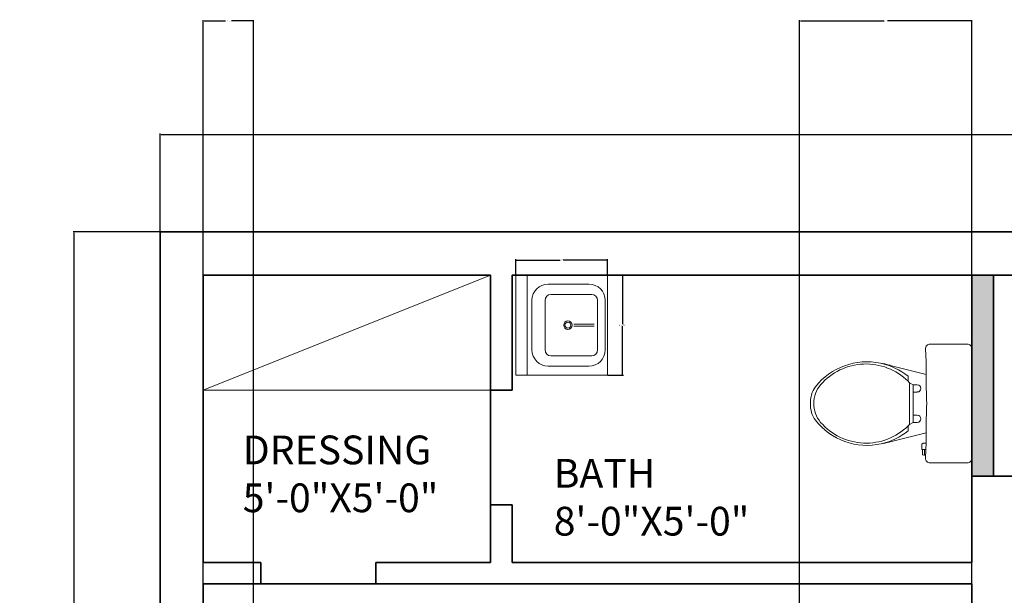
# Model space of a CAD drawing. Units: inches. Extents: x -10 to 502, y -868 to 56.
# Tile 11 of 14: x 6 to 211, y -64 to 56. Entities that reach past the tile are written whole.
import ezdxf

# ---------------------------------------------------------------- set-up
doc = ezdxf.new("R2010")
doc.units = ezdxf.units.IN
doc.header["$MEASUREMENT"] = 0
for name, color, linetype, lineweight in [('A-ANNO-DIMS', 2, 'Continuous', 18), ('A-AREA-IDEN', 7, 'Continuous', 18), ('A-FLOR-CASE', 8, 'Continuous', 18), ('A-FLOR-FIXT', 8, 'Continuous', 18), ('A-WALL', 7, 'Continuous', 35), ('A-WALL-PATT', 5, 'Continuous', 13), ('WC-Detail_dwgmodels.com', 251, 'Continuous', 13), ('WC-Outline_dwgmodels.com', 250, 'Continuous', 18)]:
    doc.layers.add(name, color=color, linetype=linetype, lineweight=lineweight)
doc.styles.get("Standard").update_dxf_attribs({"font": 'arial.ttf'})
doc.dimstyles.get("Standard").update_dxf_attribs({"dimtxt": 0.18, "dimasz": 0.18, "dimexe": 0.18, "dimexo": 0.0625, "dimgap": 0.09, "dimtad": 0, "dimtih": 1, "dimtoh": 1, "dimdec": 0, "dimzin": 0, "dimdsep": 46, "dimlunit": 3, "dimtxsty": 'Standard', "dimcen": 0.09, "dimadec": 0, "dimazin": 0, "dimtfac": 1, "dimtdec": 0, "dimtofl": 0, "dimtmove": 0, "dimatfit": 3, "dimfxl": 1, "dimtolj": 1, "dimtzin": 0, "dimarcsym": 0})

# ---------------------------------------------------------------- blocks, each defined once
blk = doc.blocks.new('*D1')
at = {"layer": 'A-ANNO-DIMS', "color": 0, "lineweight": -2, "transparency": 16777216}
for p, q in [((34.95, 12.21), (34.95, 32.67)), ((35.13, 32.49), (236.06, 32.49)), ((457.77, 32.49), (256.84, 32.49)), ((457.95, 12.21), (457.95, 32.67))]:
    blk.add_line(p, q, dxfattribs=at)
at = {"layer": 'A-ANNO-DIMS', "color": 0, "transparency": 16777216}
for points in [[(35.13, 32.52), (35.13, 32.46), (34.95, 32.49)], [(457.77, 32.52), (457.77, 32.46), (457.95, 32.49)]]:
    blk.add_solid(points, dxfattribs=at)
at = {"layer": 'Defpoints', "color": 0, "transparency": 16777216}
for p in [(457.95, 32.49), (34.95, 12.15), (457.95, 12.15)]:
    blk.add_point(p, dxfattribs=at)
at = {"layer": 'A-ANNO-DIMS', "color": 0, "transparency": 16777216, "insert": (246.45, 32.49), "char_height": 6, "attachment_point": 5}
blk.add_mtext('\\A1;35\'-3"', dxfattribs=at)
blk = doc.blocks.new('*D2')
at = {"layer": 'A-ANNO-DIMS', "color": 0, "lineweight": -2, "transparency": 16777216}
for p, q in [((34.89, 12.15), (16.75, 12.15)), ((16.93, 11.97), (16.93, -376.2)), ((16.93, -770.67), (16.93, -382.51)), ((34.89, -770.85), (16.75, -770.85))]:
    blk.add_line(p, q, dxfattribs=at)
at = {"layer": 'A-ANNO-DIMS', "color": 0, "transparency": 16777216}
for points in [[(16.9, 11.97), (16.96, 11.97), (16.93, 12.15)], [(16.9, -770.67), (16.96, -770.67), (16.93, -770.85)]]:
    blk.add_solid(points, dxfattribs=at)
at = {"layer": 'Defpoints', "color": 0, "transparency": 16777216}
for p in [(34.95, 12.15), (16.93, -770.85), (34.95, -770.85)]:
    blk.add_point(p, dxfattribs=at)
at = {"layer": 'A-ANNO-DIMS', "color": 0, "transparency": 16777216, "insert": (16.93, -379.35), "char_height": 6, "attachment_point": 5}
blk.add_mtext('\\A1;65\'-3"', dxfattribs=at)
blk = doc.blocks.new('М14 600х655')
for p, q in [((-655, 600), (-655, 0)), ((-655, 600), (-655, 0)), ((-655, 0), (-655, 600)), ((0, 600), (-655, 600)), ((0, 0), (0, 600)), ((0, 525), (-655, 525)), ((-165.1, 494.1), (-489.9, 494.1)), ((-595.8, 388.1), (-595.8, 121.3)), ((-165.4, 408.4), (-490.2, 408.4)), ((-59.2, 121.3), (-59.2, 388.1)), ((-528.4, 370.1), (-528.4, 103.3)), ((-127.2, 103.3), (-127.2, 370.1)), ((-333.5, 87.1), (-333.5, 219.6)), ((-321.5, 87.1), (-321.5, 219.6)), ((-490.2, 65.1), (-165.4, 65.1)), ((-655, 0), (-655, 0)), ((-655, 0), (-655, 0)), ((-655, 0), (0, 0)), ((-655, 0), (0, 0)), ((-489.9, 15.4), (-165.1, 15.4))]:
    blk.add_line(p, q)
for radius in [27.6, 19.3]:
    blk.add_circle((-327.5, 258.9), radius)
for centre, radius, start, end in [((-489.9, 388.1), 105.9, 90, 180), ((-165.1, 388.1), 105.9, 0, 90), ((-490.2, 370.1), 38.2, 90, 180), ((-165.4, 370.1), 38.2, 0, 90), ((-489.9, 121.3), 105.9, 180, 270), ((-490.2, 103.3), 38.2, 180, 270), ((-165.4, 103.3), 38.2, 270, 0), ((-165.1, 121.3), 105.9, 270, 0)]:
    blk.add_arc(centre, radius, start, end)
blk = doc.blocks.new('*D29')
at = {"layer": 'A-ANNO-DIMS', "color": 0, "lineweight": -2, "transparency": 16777216}
for p, q in [((128.41, 3.15), (131.66, 3.15)), ((131.48, 2.97), (131.48, -7.12)), ((131.48, -17.58), (131.48, -7.49)), ((128.41, -17.76), (131.66, -17.76))]:
    blk.add_line(p, q, dxfattribs=at)
at = {"layer": 'A-ANNO-DIMS', "color": 0, "transparency": 16777216}
for points in [[(131.45, 2.97), (131.51, 2.97), (131.48, 3.15)], [(131.45, -17.58), (131.51, -17.58), (131.48, -17.76)]]:
    blk.add_solid(points, dxfattribs=at)
at = {"layer": 'Defpoints', "color": 0, "transparency": 16777216}
for p in [(128.35, 3.15), (131.48, 3.15), (128.35, -17.76)]:
    blk.add_point(p, dxfattribs=at)
at = {"layer": 'A-ANNO-DIMS', "color": 0, "transparency": 16777216, "insert": (131.48, -7.31), "char_height": 0.18, "attachment_point": 5}
blk.add_mtext('\\A1;BASIN 1\'-9"', dxfattribs=at)
blk = doc.blocks.new('*D30')
at = {"layer": 'A-ANNO-DIMS', "color": 0, "lineweight": -2, "transparency": 16777216}
for p, q in [((109.2, 3.21), (109.2, 6.46)), ((109.38, 6.28), (118.45, 6.28)), ((128.17, 6.28), (119.09, 6.28)), ((128.35, 3.21), (128.35, 6.46))]:
    blk.add_line(p, q, dxfattribs=at)
at = {"layer": 'A-ANNO-DIMS', "color": 0, "transparency": 16777216}
for points in [[(109.38, 6.31), (109.38, 6.25), (109.2, 6.28)], [(128.17, 6.31), (128.17, 6.25), (128.35, 6.28)]]:
    blk.add_solid(points, dxfattribs=at)
at = {"layer": 'Defpoints', "color": 0, "transparency": 16777216}
for p in [(109.2, 6.28), (109.2, 3.15), (128.35, 3.15)]:
    blk.add_point(p, dxfattribs=at)
at = {"layer": 'A-ANNO-DIMS', "color": 0, "transparency": 16777216, "insert": (118.77, 6.28), "char_height": 0.18, "attachment_point": 5}
blk.add_mtext('\\A1;1\'-7"', dxfattribs=at)
blk = doc.blocks.new('*D60')
at = {"layer": 'A-ANNO-DIMS', "color": 0, "lineweight": -2, "transparency": 16777216}
for p, q in [((168.45, -332.79), (168.45, 56.38)), ((168.63, 56.2), (186.12, 56.2)), ((204.27, 56.2), (186.78, 56.2)), ((204.45, -332.79), (204.45, 56.38))]:
    blk.add_line(p, q, dxfattribs=at)
at = {"layer": 'A-ANNO-DIMS', "color": 0, "transparency": 16777216}
for points in [[(168.63, 56.23), (168.63, 56.17), (168.45, 56.2)], [(204.27, 56.23), (204.27, 56.17), (204.45, 56.2)]]:
    blk.add_solid(points, dxfattribs=at)
at = {"layer": 'Defpoints', "color": 0, "transparency": 16777216}
for p in [(204.45, 56.2), (168.45, -332.85), (204.45, -332.85)]:
    blk.add_point(p, dxfattribs=at)
at = {"layer": 'A-ANNO-DIMS', "color": 0, "transparency": 16777216, "insert": (186.45, 56.2), "char_height": 0.18, "attachment_point": 5}
blk.add_mtext('\\A1;3\'-0"', dxfattribs=at)
blk = doc.blocks.new('*D64')
at = {"layer": 'A-ANNO-DIMS', "color": 0, "lineweight": -2, "transparency": 16777216}
for p, q in [((43.95, -332.79), (43.95, 56.38)), ((44.13, 56.2), (48.59, 56.2)), ((54.27, 56.2), (49.81, 56.2)), ((54.45, -332.79), (54.45, 56.38))]:
    blk.add_line(p, q, dxfattribs=at)
at = {"layer": 'A-ANNO-DIMS', "color": 0, "transparency": 16777216}
for points in [[(44.13, 56.23), (44.13, 56.17), (43.95, 56.2)], [(54.27, 56.23), (54.27, 56.17), (54.45, 56.2)]]:
    blk.add_solid(points, dxfattribs=at)
at = {"layer": 'Defpoints', "color": 0, "transparency": 16777216}
for p in [(54.45, 56.2), (43.95, -332.85), (54.45, -332.85)]:
    blk.add_point(p, dxfattribs=at)
at = {"layer": 'A-ANNO-DIMS', "color": 0, "transparency": 16777216, "insert": (49.2, 56.2), "char_height": 0.18, "attachment_point": 5}
blk.add_mtext('\\A1;0\'-10 1/2"', dxfattribs=at)

msp = doc.modelspace()

# ---------------------------------------------------------------- hatches: boundary and pattern name
at = {"layer": 'A-WALL-PATT'}
h = msp.add_hatch(color=256, dxfattribs=at)
h.dxf.hatch_style = 1
h.paths.add_polyline_path([(208.95, 3.15), (204.45, 3.15), (204.45, -38.85), (208.95, -38.85)])

# ---------------------------------------------------------------- linework, layer by layer
at = {"layer": 'A-FLOR-CASE'}
for p, q in [((103.95, 3.15), (43.95, -20.85)), ((43.95, -20.85), (103.95, -20.85))]:
    msp.add_line(p, q, dxfattribs=at)
at = {"layer": 'A-WALL'}
for p, q in [((34.95, 12.15), (34.95, -770.85)), ((34.95, 12.15), (457.95, 12.15)), ((43.95, 3.15), (43.95, -56.85)), ((43.95, 3.15), (103.95, 3.15)), ((103.95, 3.15), (103.95, -56.85)), ((108.45, 3.15), (108.45, -20.85)), ((108.45, 3.15), (213.45, 3.15)), ((204.45, 3.15), (204.45, -56.85)), ((208.95, 3.15), (208.95, -38.85)), ((103.95, -20.85), (108.45, -20.85)), ((208.95, -38.85), (204.45, -38.85)), ((208.95, -38.85), (457.95, -38.85)), ((108.45, -44.85), (103.95, -44.85)), ((108.45, -44.85), (108.45, -56.85)), ((43.95, -56.85), (55.95, -56.85)), ((55.95, -56.85), (55.95, -61.35)), ((79.95, -56.85), (79.95, -61.35)), ((79.95, -56.85), (103.95, -56.85)), ((108.45, -56.85), (204.45, -56.85)), ((43.95, -61.35), (204.45, -61.35)), ((43.95, -61.35), (43.95, -254.85)), ((204.45, -61.35), (204.45, -227.85))]:
    msp.add_line(p, q, dxfattribs=at)
at = {"layer": 'WC-Detail_dwgmodels.com'}
for p, q in [((191.42, -19.34), (192.19, -19.76)), ((192.19, -19.76), (193.03, -19.76)), ((192.19, -21.27), (192.19, -19.76)), ((193.03, -21.27), (192.19, -21.27)), ((192.19, -23.68), (192.19, -21.27)), ((192.19, -23.68), (192.19, -26.1)), ((192.19, -26.1), (192.19, -27.6)), ((193.03, -26.1), (192.19, -26.1)), ((191.42, -28.02), (192.19, -27.6)), ((192.19, -27.6), (193.03, -27.6))]:
    msp.add_line(p, q, dxfattribs=at)
for points in [[(191.1, -19.02, 0.434217), (172.85, -19.76, 0.182634), (171.42, -23.68, 2.693815)], [(191.1, -17.97, 0.117999), (185.33, -15.25, 0.16845)], [(191.1, -19.02), (191.1, -17.97, 0.416606)], [(191.42, -19.34, 0.008985), (191.1, -19.02, 0.182634)], [(191.42, -23.68), (191.42, -19.34, 0.444938)], [(191.1, -28.34, -0.434217), (172.85, -27.6, -0.182634), (171.42, -23.68, -2.693815)], [(191.42, -23.68), (191.42, -28.02, -0.008985)], [(191.42, -28.02, -0.008985), (191.1, -28.34, -0.182634)], [(191.1, -28.34), (191.1, -29.39, -0.416606)], [(191.1, -29.39, -0.114632), (185.51, -32.08, -0.16845)]]:
    msp.add_lwpolyline(points, format="xyb", dxfattribs=at)
for centre in [(193.03, -20.51), (193.03, -26.85)]:
    msp.add_arc(centre, 0.753, 270, 90, dxfattribs=at)
at = {"layer": 'WC-Outline_dwgmodels.com'}
for points in [[(194.86, -17.59, -0.00511), (194.87, -14.87), (194.75, -12.28, -0.426005), (195.72, -11.27), (203.48, -11.27, -0.414214), (204.45, -12.24), (204.45, -23.68)], [(185.33, -15.25, 0.284616), (171.76, -20.18, 0.171216), (170.74, -23.68, 2.912347)], [(185.33, -15.25, -0.0272), (187.15, -15.63, -0.005151), (187.4, -15.7, -0.103607)], [(195.02, -23.66, -0.010344), (194.86, -17.59)], [(185.51, -32.08, -0.288211), (171.76, -27.18, -0.171216), (170.74, -23.68, -2.912232)], [(194.82, -33.26), (194.75, -35.07, 0.426005), (195.72, -36.08), (203.48, -36.08, 0.414214), (204.45, -35.11), (204.45, -23.68)], [(195.02, -23.69, 0.010344), (194.86, -29.76)], [(194.86, -29.76, 0.006773), (194.87, -31.81), (194.86, -31.97, 0.55454)], [(187.4, -31.65, -0.005151), (187.15, -31.72, -0.024565), (185.51, -32.08, -0.065413)], [(194.1, -33.26), (194.07, -33.26, -0.414214), (193.96, -33.16), (193.96, -32.29, -0.414214), (194.28, -31.97), (194.86, -31.97)], [(194.86, -31.97), (194.82, -33.26, 0.319616)], [(194.1, -33.26), (194.1, -34.29, 0.3351), (194.18, -34.39), (194.42, -34.46, 0.498015), (194.51, -34.39), (194.51, -33.26)]]:
    msp.add_lwpolyline(points, format="xyb", dxfattribs=at)
for points in [[(187.4, -15.7), (194.86, -17.59)], [(187.4, -31.65), (194.86, -29.76)], [(194.51, -33.26), (194.1, -33.26)], [(194.82, -33.26), (194.51, -33.26)]]:
    msp.add_lwpolyline(points, dxfattribs=at)

# ---------------------------------------------------------------- block references
at = {"layer": 'A-FLOR-FIXT', "xscale": 0.0319169208114052, "yscale": 0.0319169208114052, "zscale": 0.0319169208114052, "rotation": 90}
msp.add_blockref('М14 600х655', (128.35, 3.15), dxfattribs=at)

# ---------------------------------------------------------------- texts
at = {"layer": 'A-AREA-IDEN', "insert": (52.19, -30.36), "char_height": 6, "attachment_point": 1}
msp.add_mtext_dynamic_manual_height_columns('DRESSING\\P5\'-0"X5\'-0"', width=0.1346, gutter_width=1, heights=[0], dxfattribs=at)
at = {"layer": 'A-AREA-IDEN', "insert": (117.12, -35.24), "char_height": 6, "attachment_point": 1}
msp.add_mtext('BATH\\P8\'-0"X5\'-0"', dxfattribs=at)

# ---------------------------------------------------------------- dimensions: what is measured, and where the dimension line sits
at = {"layer": 'A-ANNO-DIMS'}
for base, p1, p2, override, picture, middle in [((54.45, 56.2), (43.95, -332.85), (54.45, -332.85), {"dimdec": 1, "dimlfac": 1, "dimrnd": 0, "dimzin": 1, "dimdsep": 46, "dimlunit": 4, "dimfrac": 2}, '*D64', (49.2, 56.2)), ((204.45, 56.2), (168.45, -332.85), (204.45, -332.85), {"dimdec": 1, "dimlfac": 1, "dimrnd": 0, "dimzin": 1, "dimdsep": 46, "dimlunit": 4, "dimfrac": 2}, '*D60', (186.45, 56.2)), ((457.95, 32.49), (34.95, 12.15), (457.95, 12.15), {"dimtxt": 6, "dimclrd": 0, "dimclre": 0, "dimclrt": 0}, '*D1', (246.45, 32.49))]:
    dim = msp.add_linear_dim(base=base, p1=p1, p2=p2, dimstyle='Standard', override=override, dxfattribs=at)
    dim.commit()
    dim.dimension.update_dxf_attribs({"geometry": picture, "text_midpoint": middle})
for base, p1, p2, angle, override, picture, middle in [((16.93, -770.85), (34.95, 12.15), (34.95, -770.85), 90, {"dimtxt": 6, "dimclrd": 0, "dimclre": 0, "dimclrt": 0}, '*D2', (16.93, -379.35)), ((109.1973, 6.2831), (128.3474, 3.1473), (109.1973, 3.1473), 180, {"dimdec": 1, "dimlfac": 1, "dimrnd": 0, "dimzin": 1, "dimdsep": 46, "dimlunit": 4, "dimfrac": 2}, '*D30', (118.7723, 6.2831))]:
    dim = msp.add_linear_dim(base=base, p1=p1, p2=p2, angle=angle, dimstyle='Standard', override=override, dxfattribs=at)
    dim.commit()
    dim.dimension.update_dxf_attribs({"geometry": picture, "text_midpoint": middle})
dim = msp.add_linear_dim(base=(131.48, 3.15), p1=(128.35, -17.76), p2=(128.35, 3.15), angle=90, text='BASIN <>', dimstyle='Standard', override={"dimdec": 1, "dimlfac": 1, "dimrnd": 0, "dimzin": 1, "dimdsep": 46, "dimlunit": 4, "dimfrac": 2}, dxfattribs=at)
dim.commit()
dim.dimension.update_dxf_attribs({"geometry": '*D29', "text_midpoint": (131.48, -7.31)})

doc.saveas('drawing.dxf')
